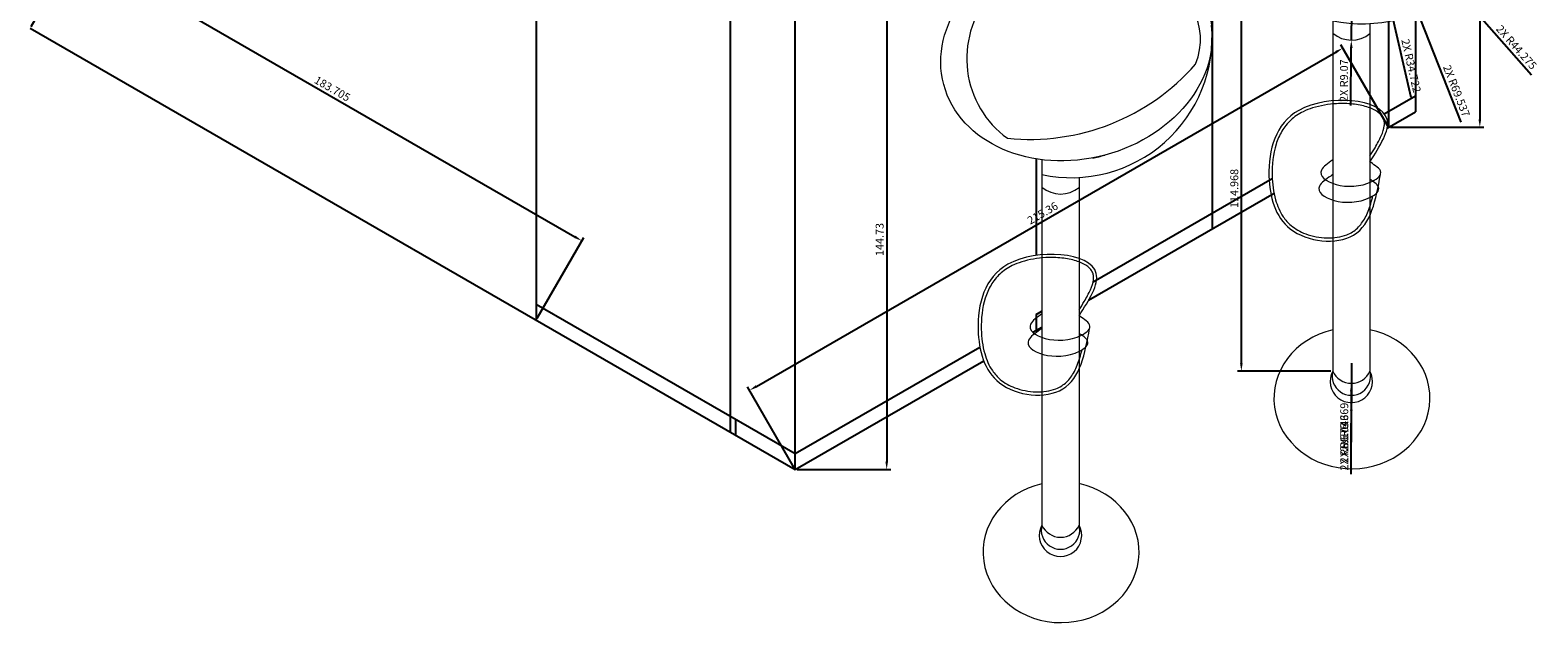
# Model space of a CAD drawing. Units: centimetres. Extents: x 239489 to 240034, y 95136 to 95693.
# Tile 1 of 4: x 239559 to 240034, y 95136 to 95322. Entities that reach past the tile are written whole.
import ezdxf

# ---------------------------------------------------------------- set-up
doc = ezdxf.new("R2010")
doc.units = ezdxf.units.CM
for name, color, linetype, lineweight in [('A-ANNO-DIMS', 2, 'Continuous', 18), ('A-FLOR-CASE', 7, 'Continuous', 25), ('A-FURN', 8, 'Continuous', 18)]:
    doc.layers.add(name, color=color, linetype=linetype, lineweight=lineweight)
doc.styles.get("Standard").update_dxf_attribs({"font": 'arial.ttf'})
doc.dimstyles.new('ISO-25', dxfattribs={"dimtxt": 2.5, "dimasz": 2.5, "dimexe": 1.25, "dimexo": 0.625, "dimtad": 1, "dimdec": 1, "dimdsep": 46, "dimtxsty": 'Standard', "dimcen": 2.5, "dimadec": 0, "dimazin": 0, "dimtfac": 1, "dimtdec": 1, "dimtmove": 0, "dimatfit": 3, "dimfxl": 1, "dimarcsym": 0})

# ---------------------------------------------------------------- blocks, each defined once
blk = doc.blocks.new('chair')
for p, q in [((240038.62, 95198.57), (240038.62, 95083.6)), ((240050.31, 95192.98), (240050.31, 95083.6))]:
    blk.add_line(p, q)
for centre, radius, start, end in [((240045.95, 95230.38), 30.97, 140.3765, 234.0123), ((240047.85, 95237.18), 44.27, 257.9755, 4.8871), ((240034.71, 95274.51), 69.54, 264.2585, 318.7167), ((240048.77, 95233.37), 34.72, 279.5939, 286.053), ((240044.52, 95196.85), 9.07, 229.4992, 309.6922), ((240044.46, 95080.37), 6.67, 151.0567, 28.8701), ((240044.47, 95082.04), 6.05, 165.0328, 14.894), ((240044.47, 95086.14), 6.37, 203.4476, 336.4791)]:
    blk.add_arc(centre, radius, start, end)
blk.add_ellipse((240049.51, 95233.34), major_axis=(41.76, 11.11), ratio=0.798178)
for centre, major_axis, ratio, start_param, end_param in [((240046.12, 95230.16), (41.76, 11.11), 0.649156, 5.842129, 8.285652), ((240044.64, 95075.07), (-24.53, 0), 0.903861, 4.9602, 10.762393)]:
    blk.add_ellipse(centre, major_axis=major_axis, ratio=ratio, start_param=start_param, end_param=end_param)
for points, knots in [([(240050.31, 95149.47), (240053.45, 95154.4), (240062.71, 95168.9), (240023.27, 95171.77), (240016.58, 95146.62), (240022.37, 95124.99), (240049.4, 95122.25), (240052.18, 95137.64), (240053.6, 95145.49)], [0, 0, 0, 0, 14.382035, 42.295085, 64.991841, 82.938136, 102.944135, 123.773993, 123.773993, 123.773993, 123.773993]), ([(240050.31, 95151.33), (240050.86, 95152.21), (240051.4, 95153.07), (240052.67, 95155.21), (240053.34, 95156.46), (240054.37, 95158.8), (240054.7, 95159.88), (240054.88, 95161.29), (240054.88, 95161.73), (240054.77, 95162.52), (240054.66, 95162.88), (240054.32, 95163.58), (240054.09, 95163.91), (240053.51, 95164.56), (240053.15, 95164.87), (240051.85, 95165.79), (240050.7, 95166.33), (240048.02, 95167.17), (240046.5, 95167.47), (240043.26, 95167.81), (240041.54, 95167.85), (240037.24, 95167.61), (240034.64, 95167.17), (240031.24, 95166.1), (240030.23, 95165.71), (240027.8, 95164.52), (240026.51, 95163.63), (240024.3, 95161.56), (240023.38, 95160.4), (240021.86, 95157.85), (240021.25, 95156.46), (240019.83, 95151.95), (240019.48, 95148.58), (240019.62, 95142.56), (240019.95, 95139.94), (240021.18, 95135.59), (240021.97, 95133.78), (240023.74, 95131.18), (240024.56, 95130.25), (240026.17, 95128.89), (240026.88, 95128.4), (240028.41, 95127.53), (240029.24, 95127.14), (240032.19, 95126.03), (240034.5, 95125.58), (240038.99, 95125.46), (240041.16, 95125.78), (240043.66, 95126.75), (240044.27, 95127.05), (240045.4, 95127.76), (240045.91, 95128.16), (240047.34, 95129.53), (240048.14, 95130.64), (240049.5, 95133.2), (240050.06, 95134.65), (240050.79, 95137.03), (240051.02, 95137.89), (240051.24, 95138.77)], [1.291453, 1.291453, 1.291453, 1.291453, 3.859328, 3.859328, 7.768299, 7.768299, 11.677271, 11.677271, 13.651412, 13.651412, 15.625553, 15.625553, 17.599694, 17.599694, 19.573836, 19.573836, 23.79302, 23.79302, 28.012204, 28.012204, 32.231389, 32.231389, 38.538282, 38.538282, 41.377864, 41.377864, 45.999792, 45.999792, 50.62172, 50.62172, 55.243647, 55.243647, 64.836636, 64.836636, 72.329787, 72.329787, 78.440683, 78.440683, 82.448991, 82.448991, 85.126657, 85.126657, 87.804323, 87.804323, 94.31242, 94.31242, 100.820517, 100.820517, 103.180094, 103.180094, 105.53967, 105.53967, 110.270519, 110.270519, 115.001369, 115.001369, 117.513572, 117.513572, 117.513572, 117.513572]), ([(240038.62, 95150.05), (240037.1, 95148.99), (240030.34, 95144.28), (240045.99, 95138.79), (240055.45, 95146.41), (240051.11, 95148.83), (240050.31, 95149.47)], [0, 0, 0, 0, 4.688566, 20.875909, 24.405284, 27.513147, 27.513147, 27.513147, 27.513147]), ([(240038.62, 95145.45), (240038.41, 95145.3), (240038.2, 95145.16), (240037.99, 95145.01), (240036.47, 95143.95), (240029.7, 95139.25), (240045.36, 95133.75), (240054.55, 95141.16), (240051.25, 95143.33), (240050.31, 95143.98)], [-0.650979, -0.650979, -0.650979, -0.650979, 0, 0, 0, 4.688566, 20.875909, 24.405284, 26.869866, 26.869866, 26.869866, 26.869866])]:
    blk.add_open_spline(points, degree=3, knots=knots)
blk = doc.blocks.new('*D9')
at = {"layer": 'A-ANNO-DIMS', "color": 0, "lineweight": -2, "transparency": 16777216}
for p, q in [((239987.18, 95502.44), (240016.56, 95502.44)), ((240015.31, 95499.94), (240015.31, 95294.12)), ((239987.18, 95291.62), (240016.56, 95291.62))]:
    blk.add_line(p, q, dxfattribs=at)
at = {"layer": 'A-ANNO-DIMS', "color": 0, "transparency": 16777216}
for points in [[(240014.89, 95499.94), (240015.73, 95499.94), (240015.31, 95502.44)], [(240014.89, 95294.12), (240015.73, 95294.12), (240015.31, 95291.62)]]:
    blk.add_solid(points, dxfattribs=at)
at = {"layer": 'Defpoints', "color": 0, "transparency": 16777216}
for p in [(239986.56, 95502.44), (239986.56, 95291.62), (240015.31, 95291.62)]:
    blk.add_point(p, dxfattribs=at)
at = {"layer": 'A-ANNO-DIMS', "color": 0, "transparency": 16777216, "insert": (240013.41, 95397.03), "char_height": 2.5, "attachment_point": 5, "rotation": 90}
blk.add_mtext('210.82', dxfattribs=at)
blk = doc.blocks.new('*D11')
at = {"layer": 'A-ANNO-DIMS', "color": 0, "lineweight": -2, "transparency": 16777216}
for p, q in [((239559.76, 95323.39), (239574.45, 95348.83)), ((239575.99, 95346.5), (239730.75, 95257.15)), ((239718.86, 95231.54), (239733.54, 95256.98))]:
    blk.add_line(p, q, dxfattribs=at)
at = {"layer": 'A-ANNO-DIMS', "color": 0, "transparency": 16777216}
for points in [[(239576.2, 95346.86), (239575.78, 95346.14), (239573.83, 95347.75)], [(239730.96, 95257.51), (239730.55, 95256.79), (239732.92, 95255.9)]]:
    blk.add_solid(points, dxfattribs=at)
at = {"layer": 'Defpoints', "color": 0, "transparency": 16777216}
for p in [(239559.45, 95322.85), (239732.92, 95255.9), (239718.54, 95231)]:
    blk.add_point(p, dxfattribs=at)
at = {"layer": 'A-ANNO-DIMS', "color": 0, "transparency": 16777216, "insert": (239654.32, 95303.47), "char_height": 2.5, "attachment_point": 5, "rotation": 330}
blk.add_mtext('183.705', dxfattribs=at)
blk = doc.blocks.new('*D42')
at = {"layer": 'A-ANNO-DIMS', "color": 0, "lineweight": -2, "transparency": 16777216}
for p, q in [((239800.67, 95328.67), (239830.05, 95328.67)), ((239828.8, 95326.17), (239828.8, 95186.44)), ((239800.67, 95183.94), (239830.05, 95183.94))]:
    blk.add_line(p, q, dxfattribs=at)
at = {"layer": 'A-ANNO-DIMS', "color": 0, "transparency": 16777216}
for points in [[(239828.38, 95326.17), (239829.22, 95326.17), (239828.8, 95328.67)], [(239828.38, 95186.44), (239829.22, 95186.44), (239828.8, 95183.94)]]:
    blk.add_solid(points, dxfattribs=at)
at = {"layer": 'Defpoints', "color": 0, "transparency": 16777216}
for p in [(239800.05, 95328.67), (239800.05, 95183.94), (239828.8, 95183.94)]:
    blk.add_point(p, dxfattribs=at)
at = {"layer": 'A-ANNO-DIMS', "color": 0, "transparency": 16777216, "insert": (239826.9, 95256.31), "char_height": 2.5, "attachment_point": 5, "rotation": 90}
blk.add_mtext('144.73', dxfattribs=at)
blk = doc.blocks.new('*D43')
at = {"layer": 'A-ANNO-DIMS', "color": 0, "lineweight": -2, "transparency": 16777216}
for p, q in [((239787.84, 95210.09), (239970.02, 95315.27)), ((239986.25, 95292.16), (239971.56, 95317.6)), ((239799.74, 95184.48), (239785.05, 95209.92))]:
    blk.add_line(p, q, dxfattribs=at)
at = {"layer": 'A-ANNO-DIMS', "color": 0, "transparency": 16777216}
for points in [[(239969.81, 95315.63), (239970.23, 95314.91), (239972.18, 95316.52)], [(239787.63, 95210.45), (239788.05, 95209.73), (239785.67, 95208.84)]]:
    blk.add_solid(points, dxfattribs=at)
at = {"layer": 'Defpoints', "color": 0, "transparency": 16777216}
for p in [(239972.18, 95316.52), (239986.56, 95291.62), (239800.05, 95183.94)]:
    blk.add_point(p, dxfattribs=at)
at = {"layer": 'A-ANNO-DIMS', "color": 0, "transparency": 16777216, "insert": (239877.98, 95264.33), "char_height": 2.5, "attachment_point": 5, "rotation": 30}
blk.add_mtext('215.36', dxfattribs=at)
blk = doc.blocks.new('*D47')
at = {"layer": 'A-ANNO-DIMS', "color": 0, "lineweight": -2, "transparency": 16777216}
for p, q in [((239968.45, 95329.85), (239939.07, 95329.85)), ((239940.32, 95217.39), (239940.32, 95327.35)), ((239968.45, 95214.89), (239939.07, 95214.89))]:
    blk.add_line(p, q, dxfattribs=at)
at = {"layer": 'A-ANNO-DIMS', "color": 0, "transparency": 16777216}
for points in [[(239939.91, 95327.35), (239940.74, 95327.35), (239940.32, 95329.85)], [(239939.91, 95217.39), (239940.74, 95217.39), (239940.32, 95214.89)]]:
    blk.add_solid(points, dxfattribs=at)
at = {"layer": 'Defpoints', "color": 0, "transparency": 16777216}
for p in [(239940.32, 95329.85), (239969.07, 95329.85), (239969.07, 95214.89)]:
    blk.add_point(p, dxfattribs=at)
at = {"layer": 'A-ANNO-DIMS', "color": 0, "transparency": 16777216, "insert": (239938.42, 95272.37), "char_height": 2.5, "attachment_point": 5, "rotation": 90}
blk.add_mtext('114.968', dxfattribs=at)
blk = doc.blocks.new('*D52')
at = {"layer": 'A-ANNO-DIMS', "color": 0, "lineweight": -2, "transparency": 16777216}
for p, q in [((239965.16, 95405.79), (239990.63, 95341.09)), ((240009.47, 95293.22), (239991.54, 95338.76))]:
    blk.add_line(p, q, dxfattribs=at)
at = {"layer": 'A-ANNO-DIMS', "color": 0, "transparency": 16777216}
blk.add_solid([(239991.93, 95338.91), (239991.16, 95338.61), (239990.63, 95341.09)], dxfattribs=at)
at = {"layer": 'Defpoints', "color": 0, "transparency": 16777216}
for p in [(239965.16, 95405.79), (239990.63, 95341.09)]:
    blk.add_point(p, dxfattribs=at)
at = {"layer": 'A-ANNO-DIMS', "color": 0, "transparency": 16777216, "insert": (240007.68, 95302.96), "char_height": 2.5, "attachment_point": 5, "rotation": 291.4873}
blk.add_mtext('2X R69.537', dxfattribs=at)
blk = doc.blocks.new('*D53')
at = {"layer": 'A-ANNO-DIMS', "color": 0, "lineweight": -2, "transparency": 16777216}
for p, q in [((239978.3, 95368.47), (240007.59, 95335.27)), ((240031.61, 95308.06), (240009.25, 95333.4))]:
    blk.add_line(p, q, dxfattribs=at)
at = {"layer": 'A-ANNO-DIMS', "color": 0, "transparency": 16777216}
blk.add_solid([(240009.56, 95333.67), (240008.94, 95333.12), (240007.59, 95335.27)], dxfattribs=at)
at = {"layer": 'Defpoints', "color": 0, "transparency": 16777216}
for p in [(239978.3, 95368.47), (240007.59, 95335.27)]:
    blk.add_point(p, dxfattribs=at)
at = {"layer": 'A-ANNO-DIMS', "color": 0, "transparency": 16777216, "insert": (240026.6, 95316.61), "char_height": 2.5, "attachment_point": 5, "rotation": 311.4309}
blk.add_mtext('2X R44.275', dxfattribs=at)
blk = doc.blocks.new('*D54')
at = {"layer": 'A-ANNO-DIMS', "color": 0, "lineweight": -2, "transparency": 16777216}
for p, q in [((239979.22, 95364.65), (239986.93, 95330.8)), ((239993.71, 95301.02), (239987.48, 95328.36))]:
    blk.add_line(p, q, dxfattribs=at)
at = {"layer": 'A-ANNO-DIMS', "color": 0, "transparency": 16777216}
blk.add_solid([(239987.89, 95328.45), (239987.08, 95328.27), (239986.93, 95330.8)], dxfattribs=at)
at = {"layer": 'Defpoints', "color": 0, "transparency": 16777216}
for p in [(239979.22, 95364.65), (239986.93, 95330.8)]:
    blk.add_point(p, dxfattribs=at)
at = {"layer": 'A-ANNO-DIMS', "color": 0, "transparency": 16777216, "insert": (239993.41, 95310.91), "char_height": 2.5, "attachment_point": 5, "rotation": 282.8235}
blk.add_mtext('2X R34.722', dxfattribs=at)
blk = doc.blocks.new('*D56')
at = {"layer": 'A-ANNO-DIMS', "color": 0, "lineweight": -2, "transparency": 16777216}
for p, q in [((239974.96, 95328.13), (239974.9, 95319.06)), ((239974.75, 95298.51), (239974.88, 95316.56))]:
    blk.add_line(p, q, dxfattribs=at)
at = {"layer": 'A-ANNO-DIMS', "color": 0, "transparency": 16777216}
blk.add_solid([(239974.46, 95316.57), (239975.3, 95316.56), (239974.9, 95319.06)], dxfattribs=at)
at = {"layer": 'Defpoints', "color": 0, "transparency": 16777216}
for p in [(239974.96, 95328.13), (239974.9, 95319.06)]:
    blk.add_point(p, dxfattribs=at)
at = {"layer": 'A-ANNO-DIMS', "color": 0, "transparency": 16777216, "insert": (239972.91, 95306.3), "char_height": 2.5, "attachment_point": 5, "rotation": 89.593}
blk.add_mtext('2X R9.07', dxfattribs=at)
blk = doc.blocks.new('*D57')
at = {"layer": 'A-ANNO-DIMS', "color": 0, "lineweight": -2, "transparency": 16777216}
for p, q in [((239974.91, 95211.66), (239974.91, 95204.98)), ((239974.89, 95182.49), (239974.91, 95202.48))]:
    blk.add_line(p, q, dxfattribs=at)
at = {"layer": 'A-ANNO-DIMS', "color": 0, "transparency": 16777216}
blk.add_solid([(239974.49, 95202.48), (239975.32, 95202.48), (239974.91, 95204.98)], dxfattribs=at)
at = {"layer": 'Defpoints', "color": 0, "transparency": 16777216}
for p in [(239974.91, 95211.66), (239974.91, 95204.98)]:
    blk.add_point(p, dxfattribs=at)
at = {"layer": 'A-ANNO-DIMS', "color": 0, "transparency": 16777216, "insert": (239973, 95191.24), "char_height": 2.5, "attachment_point": 5, "rotation": 89.9622}
blk.add_mtext('2X R6.673', dxfattribs=at)
blk = doc.blocks.new('*D58')
at = {"layer": 'A-ANNO-DIMS', "color": 0, "lineweight": -2, "transparency": 16777216}
for p, q in [((239974.92, 95217.42), (239974.91, 95211.05)), ((239974.9, 95188.55), (239974.91, 95208.55))]:
    blk.add_line(p, q, dxfattribs=at)
at = {"layer": 'A-ANNO-DIMS', "color": 0, "transparency": 16777216}
blk.add_solid([(239974.49, 95208.55), (239975.33, 95208.55), (239974.91, 95211.05)], dxfattribs=at)
at = {"layer": 'Defpoints', "color": 0, "transparency": 16777216}
for p in [(239974.92, 95217.42), (239974.91, 95211.05)]:
    blk.add_point(p, dxfattribs=at)
at = {"layer": 'A-ANNO-DIMS', "color": 0, "transparency": 16777216, "insert": (239973, 95197.3), "char_height": 2.5, "attachment_point": 5, "rotation": 89.9632}
blk.add_mtext('2X R6.369', dxfattribs=at)
blk = doc.blocks.new('*D59')
at = {"layer": 'A-ANNO-DIMS', "color": 0, "lineweight": -2, "transparency": 16777216}
for p, q in [((239974.91, 95213.32), (239974.91, 95207.28)), ((239974.9, 95184.79), (239974.91, 95204.78))]:
    blk.add_line(p, q, dxfattribs=at)
at = {"layer": 'A-ANNO-DIMS', "color": 0, "transparency": 16777216}
blk.add_solid([(239974.49, 95204.78), (239975.33, 95204.78), (239974.91, 95207.28)], dxfattribs=at)
at = {"layer": 'Defpoints', "color": 0, "transparency": 16777216}
for p in [(239974.91, 95213.32), (239974.91, 95207.28)]:
    blk.add_point(p, dxfattribs=at)
at = {"layer": 'A-ANNO-DIMS', "color": 0, "transparency": 16777216, "insert": (239973, 95193.53), "char_height": 2.5, "attachment_point": 5, "rotation": 89.9671}
blk.add_mtext('2X R6.046', dxfattribs=at)

msp = doc.modelspace()

# ---------------------------------------------------------------- linework, layer by layer
at = {"layer": 'A-FLOR-CASE'}
for p, q in [((239931.1756, 95404.3778), (239931.1756, 95259.6464)), ((239718.5446, 95375.7293), (239718.5446, 95230.9978)), ((239779.6981, 95195.6908), (239779.6981, 95340.4222)), ((239800.0497, 95183.9408), (239800.0497, 95328.6722)), ((239986.5584, 95324.9711), (239986.5584, 95291.6216)), ((239995.0624, 95327.4906), (239995.0624, 95296.5314)), ((239559.4517, 95322.8502), (239800.0497, 95183.9408)), ((239985.26, 95295.872), (239995.0624, 95301.5314)), ((239986.1669, 95291.3956), (239995.0624, 95296.5314)), ((239875.7928, 95281.6735), (239875.7928, 95251.3068)), ((239893.6961, 95243.0076), (239950.041, 95275.5383)), ((239892.2988, 95237.2008), (239950.5903, 95270.8555)), ((239718.5446, 95235.9978), (239800.0497, 95188.9408)), ((239875.7928, 95232.6711), (239877.6125, 95233.7217)), ((239874.8023, 95227.0992), (239877.6125, 95228.7217)), ((239875.7928, 95232.6711), (239875.7928, 95227.6711)), ((239800.0497, 95188.9408), (239858.1032, 95222.458)), ((239800.0497, 95183.9408), (239859.3024, 95218.1504)), ((239781.3086, 95194.761), (239781.3086, 95199.761))]:
    msp.add_line(p, q, dxfattribs=at)

# ---------------------------------------------------------------- block references
at = {"layer": 'A-FURN'}
for p in [(-69.552, 131.2835), (-161.0124, 82.8431)]:
    msp.add_blockref('chair', p, dxfattribs=at)

# ---------------------------------------------------------------- dimensions: what is measured, and where the dimension line sits
at = {"layer": 'A-ANNO-DIMS'}
for base, p1, p2, angle, override, picture, middle in [((240015.3084, 95291.6216), (239986.5584, 95502.4404), (239986.5584, 95291.6216), 270, {"dimdec": 2, "dimlfac": 1, "dimrnd": 0, "dimzin": 0, "dimdsep": 46, "dimlunit": 2}, '*D9', (240013.407, 95397.031)), ((239732.9196, 95255.8961), (239559.4517, 95322.8502), (239718.5446, 95230.9978), 330, {"dimdec": 3, "dimlfac": 1, "dimrnd": 0, "dimzin": 0, "dimdsep": 46, "dimlunit": 2}, '*D11', (239654.3243, 95303.4697)), ((239828.7997, 95183.9408), (239800.0497, 95328.6722), (239800.0497, 95183.9408), 270, {"dimdec": 2, "dimlfac": 1, "dimrnd": 0, "dimzin": 0, "dimdsep": 46, "dimlunit": 2}, '*D42', (239826.8975, 95256.3065)), ((239940.3229, 95329.8541), (239969.0729, 95214.8863), (239969.0729, 95329.8541), 90, {"dimdec": 3, "dimlfac": 1, "dimrnd": 0, "dimzin": 0, "dimdsep": 46, "dimlunit": 2}, '*D47', (239938.4215, 95272.3702)), ((239972.1834, 95316.5199), (239800.0497, 95183.9408), (239986.5584, 95291.6216), 30, {"dimdec": 2, "dimlfac": 1, "dimrnd": 0, "dimzin": 0, "dimdsep": 46, "dimlunit": 2}, '*D43', (239877.9779, 95264.3269))]:
    dim = msp.add_linear_dim(base=base, p1=p1, p2=p2, angle=angle, dimstyle='ISO-25', override=override, dxfattribs=at)
    dim.commit()
    dim.dimension.update_dxf_attribs({"geometry": picture, "text_midpoint": middle})
for center, mpoint, picture, middle in [((239965.1581, 95405.7905), (239990.6291, 95341.0866), '*D52', (240005.9117, 95302.2643)), ((239978.2967, 95368.4682), (240007.594, 95335.273), '*D53', (240025.1724, 95315.3559)), ((239979.2226, 95364.6538), (239986.929, 95330.7982), '*D54', (239991.5528, 95310.4848))]:
    dim = msp.add_radius_dim(center=center, mpoint=mpoint, text='2X <>', dimstyle='ISO-25', override={"dimdec": 3, "dimlfac": 1, "dimrnd": 0, "dimzin": 0, "dimdsep": 46, "dimlunit": 2}, dxfattribs=at)
    dim.commit()
    dim.dimension.update_dxf_attribs({"geometry": picture, "text_midpoint": middle, "dimtype": 164})
for center, mpoint, override, picture, middle in [((239974.9634, 95328.1337), (239974.899, 95319.0641), {"dimdec": 2, "dimlfac": 1, "dimrnd": 0, "dimzin": 0, "dimdsep": 46, "dimlunit": 2}, '*D56', (239972.9069, 95306.3025)), ((239974.9161, 95217.4207), (239974.912, 95211.0516), {"dimdec": 3, "dimlfac": 1, "dimrnd": 0, "dimzin": 0, "dimdsep": 46, "dimlunit": 2}, '*D58', (239973.0009, 95197.3037)), ((239974.9124, 95211.657), (239974.908, 95204.9841), {"dimdec": 3, "dimlfac": 1, "dimrnd": 0, "dimzin": 0, "dimdsep": 46, "dimlunit": 2}, '*D57', (239972.9966, 95191.2388)), ((239974.9135, 95213.325), (239974.91, 95207.2793), {"dimdec": 3, "dimlfac": 1, "dimrnd": 0, "dimzin": 0, "dimdsep": 46, "dimlunit": 2}, '*D59', (239973.0007, 95193.5347))]:
    dim = msp.add_radius_dim(center=center, mpoint=mpoint, text='2X <>', dimstyle='ISO-25', override=override, dxfattribs=at)
    dim.commit()
    dim.dimension.update_dxf_attribs({"geometry": picture, "text_midpoint": middle})

doc.saveas('drawing.dxf')
